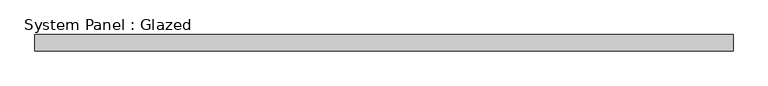
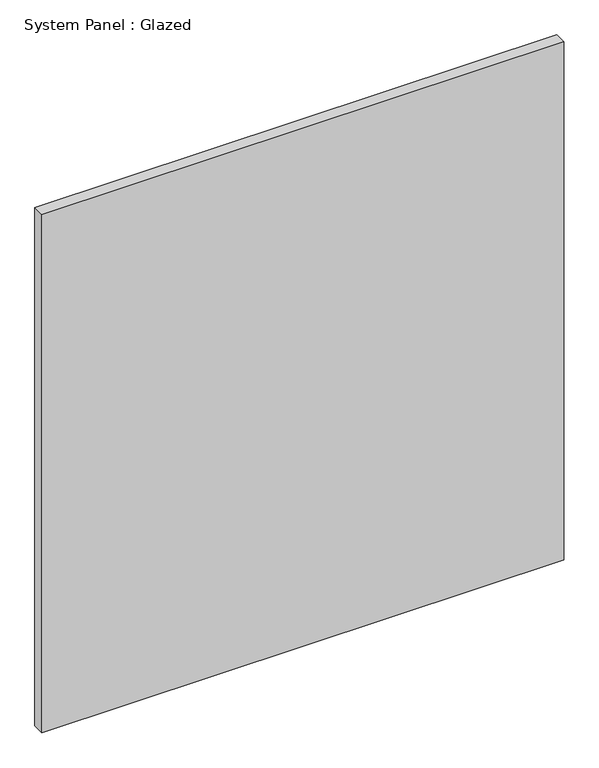
"""IFC4 building model written with IfcOpenShell, lengths in millimetres: plate geometry, System Panel : Glazed."""

from ifc_helpers import new_model, si_unit, origin, origin_with_axes, place, context, project, spatial, polyline, outline, extrude, source, transform, mapped, element, save


def system_panel_glazed_4d72b045(model_context):
    return source(origin(), model_context, "Body", "SweptSolid", [
        extrude(outline(polyline([(550.3333334, 19.05), (-550.3333334, 19.05), (-550.3333334, 44.45), (550.3333334, 44.45), (550.3333334, 19.05)])), origin_with_axes(), (0.0, 0.0, 1.0), 1155.7),
    ])


if __name__ == "__main__":
    model = new_model("IFC4")
    model_context = context("Model", 3, world=origin())
    ifc_project = project(units=[si_unit("LENGTHUNIT", "METRE", prefix="MILLI")], contexts=[model_context])
    site = spatial("IfcSite", under=ifc_project)
    building = spatial("IfcBuilding", under=site)
    placement = place(None, origin())
    system_panel_glazed_shape = system_panel_glazed_4d72b045(model_context)
    element("IfcPlate", 1, ObjectType="System Panel : Glazed", at=placement, inside=building, context=model_context, shape_type="MappedRepresentation", body=[
        mapped(system_panel_glazed_shape, transform((0.0, 0.0, 0.0), x_axis=(1.0, 0.0, 0.0), y_axis=(0.0, 1.0, 0.0), z_axis=(0.0, 0.0, 1.0))),
    ])
    save(model, "model.ifc")

# Revit data of these elements
# Type "System Panel : Glazed"
#   Construction Type Id = "GSP4R"
#   Analytic Construction = "1/8 in Pilkington single glazing"
#   Visual Light Transmittance = 0.9
#   Solar Heat Gain Coefficient = 0.86
#   Heat Transfer Coefficient (U) = 1.18115 BTU/(h·ft²·°F)
#   Define Thermal Properties by = 1
# Element 1 (IfcPlate, "System Panel : Glazed")
#   Materials on its faces: "Glass"
# Materials
#   "Glass": class "Glass", colour RGB 0 128 192, transparency 0.75, Description = "Soda Lime Glass", Cost = 0
